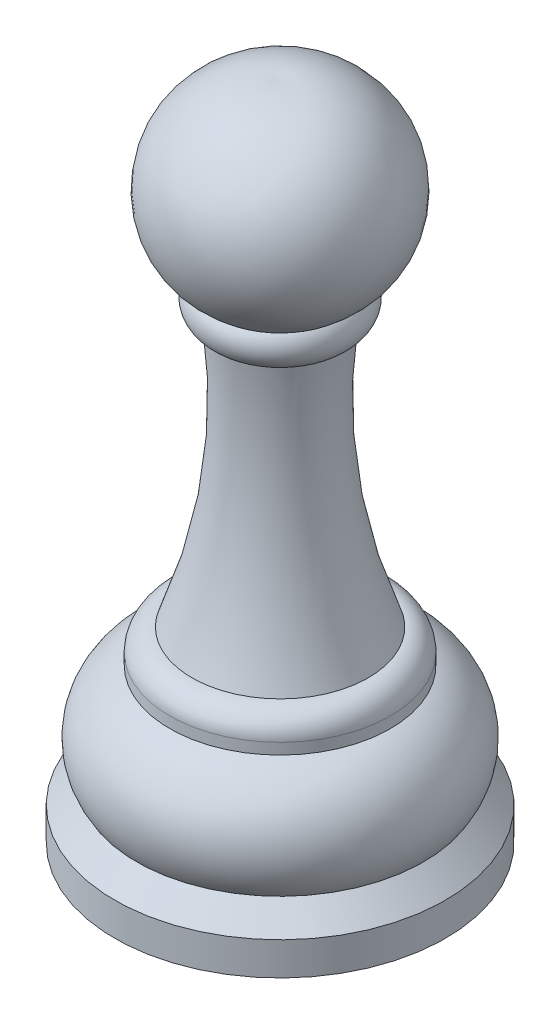
ISO-10303-21;
HEADER;
FILE_DESCRIPTION(('STEP AP214'),'2;1');
FILE_NAME('part.step','',(''),(''),'','','');
FILE_SCHEMA(('AUTOMOTIVE_DESIGN { 1 0 10303 214 1 1 1 1 }'));
ENDSEC;
DATA;
#1=APPLICATION_CONTEXT('core data for automotive mechanical design processes');
#2=APPLICATION_PROTOCOL_DEFINITION('international standard','automotive_design',2000,#1);
#3=PRODUCT_CONTEXT('',#1,'mechanical');
#4=PRODUCT('Part','Part','',(#3));
#5=PRODUCT_RELATED_PRODUCT_CATEGORY('part','',(#4));
#6=PRODUCT_DEFINITION_FORMATION('','',#4);
#7=PRODUCT_DEFINITION_CONTEXT('part definition',#1,'design');
#8=PRODUCT_DEFINITION('design','',#6,#7);
#9=PRODUCT_DEFINITION_SHAPE('','',#8);
#10=(LENGTH_UNIT() NAMED_UNIT(*) SI_UNIT(.MILLI.,.METRE.));
#11=(NAMED_UNIT(*) PLANE_ANGLE_UNIT() SI_UNIT($,.RADIAN.));
#12=(NAMED_UNIT(*) SI_UNIT($,.STERADIAN.) SOLID_ANGLE_UNIT());
#13=UNCERTAINTY_MEASURE_WITH_UNIT(LENGTH_MEASURE(1.E-05),#10,'distance_accuracy_value','');
#14=(GEOMETRIC_REPRESENTATION_CONTEXT(3) GLOBAL_UNCERTAINTY_ASSIGNED_CONTEXT((#13)) GLOBAL_UNIT_ASSIGNED_CONTEXT((#10,
#11,#12)) REPRESENTATION_CONTEXT('',''));
#15=CARTESIAN_POINT('',(0.,0.,0.));
#16=DIRECTION('',(0.,0.,1.));
#17=DIRECTION('',(1.,0.,0.));
#18=AXIS2_PLACEMENT_3D('',#15,#16,#17);
#19=CARTESIAN_POINT('',(0.,0.,0.));
#20=DIRECTION('',(0.,-1.,0.));
#21=DIRECTION('',(0.,0.,-1.));
#22=AXIS2_PLACEMENT_3D('',#19,#20,#21);
#23=PLANE('',#22);
#24=CARTESIAN_POINT('',(0.,0.,0.));
#25=DIRECTION('',(0.,-1.,0.));
#26=DIRECTION('',(0.,0.,-1.));
#27=AXIS2_PLACEMENT_3D('',#24,#25,#26);
#28=CIRCLE('',#27,15.);
#29=CARTESIAN_POINT('',(0.,0.,-15.));
#30=VERTEX_POINT('',#29);
#31=EDGE_CURVE('E11',#30,#30,#28,.T.);
#32=ORIENTED_EDGE('',*,*,#31,.T.);
#33=EDGE_LOOP('',(#32));
#34=FACE_BOUND('',#33,.T.);
#35=ADVANCED_FACE('F39',(#34),#23,.T.);
#36=CARTESIAN_POINT('',(0.,0.,0.));
#37=DIRECTION('',(0.,-1.,0.));
#38=DIRECTION('',(0.,0.,-1.));
#39=AXIS2_PLACEMENT_3D('',#36,#37,#38);
#40=CYLINDRICAL_SURFACE('',#39,15.);
#41=CARTESIAN_POINT('',(0.,3.,0.));
#42=DIRECTION('',(0.,-1.,0.));
#43=DIRECTION('',(0.,0.,-1.));
#44=AXIS2_PLACEMENT_3D('',#41,#42,#43);
#45=CIRCLE('',#44,15.);
#46=CARTESIAN_POINT('',(0.,3.,-15.));
#47=VERTEX_POINT('',#46);
#48=EDGE_CURVE('E44',#47,#47,#45,.T.);
#49=ORIENTED_EDGE('',*,*,#48,.T.);
#50=EDGE_LOOP('',(#49));
#51=FACE_BOUND('',#50,.T.);
#52=ORIENTED_EDGE('',*,*,#31,.F.);
#53=EDGE_LOOP('',(#52));
#54=FACE_BOUND('',#53,.T.);
#55=ADVANCED_FACE('F78',(#51,#54),#40,.T.);
#56=CARTESIAN_POINT('',(0.,3.,0.));
#57=DIRECTION('',(0.,-1.,0.));
#58=DIRECTION('',(0.,0.,-1.));
#59=AXIS2_PLACEMENT_3D('',#56,#57,#58);
#60=CONICAL_SURFACE('',#59,15.,0.785398163397448);
#61=CARTESIAN_POINT('',(0.,5.,0.));
#62=DIRECTION('',(0.,-1.,0.));
#63=DIRECTION('',(0.,0.,-1.));
#64=AXIS2_PLACEMENT_3D('',#61,#62,#63);
#65=CIRCLE('',#64,13.);
#66=CARTESIAN_POINT('',(0.,5.,-13.));
#67=VERTEX_POINT('',#66);
#68=EDGE_CURVE('E73',#67,#67,#65,.T.);
#69=ORIENTED_EDGE('',*,*,#68,.T.);
#70=EDGE_LOOP('',(#69));
#71=FACE_BOUND('',#70,.T.);
#72=ORIENTED_EDGE('',*,*,#48,.F.);
#73=EDGE_LOOP('',(#72));
#74=FACE_BOUND('',#73,.T.);
#75=ADVANCED_FACE('F80',(#71,#74),#60,.T.);
#76=CARTESIAN_POINT('',(0.,8.31380661428568,0.));
#77=DIRECTION('',(0.,-1.,0.));
#78=DIRECTION('',(0.,0.,-1.));
#79=AXIS2_PLACEMENT_3D('',#76,#77,#78);
#80=TOROIDAL_SURFACE('',#79,7.99813177671417,6.);
#81=CARTESIAN_POINT('',(0.,13.97,0.));
#82=DIRECTION('',(0.,-1.,0.));
#83=DIRECTION('',(0.,0.,-1.));
#84=AXIS2_PLACEMENT_3D('',#81,#82,#83);
#85=CIRCLE('',#84,10.);
#86=CARTESIAN_POINT('',(0.,13.97,-10.));
#87=VERTEX_POINT('',#86);
#88=EDGE_CURVE('E66',#87,#87,#85,.T.);
#89=ORIENTED_EDGE('',*,*,#88,.T.);
#90=EDGE_LOOP('',(#89));
#91=FACE_BOUND('',#90,.T.);
#92=ORIENTED_EDGE('',*,*,#68,.F.);
#93=EDGE_LOOP('',(#92));
#94=FACE_BOUND('',#93,.T.);
#95=ADVANCED_FACE('F83',(#91,#94),#80,.T.);
#96=CARTESIAN_POINT('',(0.,0.,0.));
#97=DIRECTION('',(0.,-1.,0.));
#98=DIRECTION('',(0.,0.,-1.));
#99=AXIS2_PLACEMENT_3D('',#96,#97,#98);
#100=CYLINDRICAL_SURFACE('',#99,10.);
#101=CARTESIAN_POINT('',(0.,14.97,0.));
#102=DIRECTION('',(0.,-1.,0.));
#103=DIRECTION('',(0.,0.,-1.));
#104=AXIS2_PLACEMENT_3D('',#101,#102,#103);
#105=CIRCLE('',#104,10.);
#106=CARTESIAN_POINT('',(0.,14.97,-10.));
#107=VERTEX_POINT('',#106);
#108=EDGE_CURVE('E64',#107,#107,#105,.T.);
#109=ORIENTED_EDGE('',*,*,#108,.T.);
#110=EDGE_LOOP('',(#109));
#111=FACE_BOUND('',#110,.T.);
#112=ORIENTED_EDGE('',*,*,#88,.F.);
#113=EDGE_LOOP('',(#112));
#114=FACE_BOUND('',#113,.T.);
#115=ADVANCED_FACE('F88',(#111,#114),#100,.T.);
#116=CARTESIAN_POINT('',(0.,14.97,0.));
#117=DIRECTION('',(0.,-1.,0.));
#118=DIRECTION('',(0.,0.,-1.));
#119=AXIS2_PLACEMENT_3D('',#116,#117,#118);
#120=TOROIDAL_SURFACE('',#119,8.,2.);
#121=CARTESIAN_POINT('',(0.,16.97,0.));
#122=DIRECTION('',(0.,-1.,0.));
#123=DIRECTION('',(0.,0.,-1.));
#124=AXIS2_PLACEMENT_3D('',#121,#122,#123);
#125=CIRCLE('',#124,8.);
#126=CARTESIAN_POINT('',(0.,16.97,-8.));
#127=VERTEX_POINT('',#126);
#128=EDGE_CURVE('E58',#127,#127,#125,.T.);
#129=ORIENTED_EDGE('',*,*,#128,.T.);
#130=EDGE_LOOP('',(#129));
#131=FACE_BOUND('',#130,.T.);
#132=ORIENTED_EDGE('',*,*,#108,.F.);
#133=EDGE_LOOP('',(#132));
#134=FACE_BOUND('',#133,.T.);
#135=ADVANCED_FACE('F123',(#131,#134),#120,.T.);
#136=CARTESIAN_POINT('',(0.,35.0019065796665,0.));
#137=DIRECTION('',(0.,-1.,0.));
#138=DIRECTION('',(0.,0.,-1.));
#139=AXIS2_PLACEMENT_3D('',#136,#137,#138);
#140=TOROIDAL_SURFACE('',#139,54.635290768925,50.);
#141=CARTESIAN_POINT('',(0.,41.03,0.));
#142=DIRECTION('',(0.,-1.,0.));
#143=DIRECTION('',(0.,0.,-1.));
#144=AXIS2_PLACEMENT_3D('',#141,#142,#143);
#145=CIRCLE('',#144,5.);
#146=CARTESIAN_POINT('',(0.,41.03,-5.));
#147=VERTEX_POINT('',#146);
#148=EDGE_CURVE('E60',#147,#147,#145,.T.);
#149=ORIENTED_EDGE('',*,*,#148,.T.);
#150=EDGE_LOOP('',(#149));
#151=FACE_BOUND('',#150,.T.);
#152=ORIENTED_EDGE('',*,*,#128,.F.);
#153=EDGE_LOOP('',(#152));
#154=FACE_BOUND('',#153,.T.);
#155=ADVANCED_FACE('F131',(#151,#154),#140,.F.);
#156=CARTESIAN_POINT('',(0.,42.966609004825,0.));
#157=DIRECTION('',(0.,-1.,0.));
#158=DIRECTION('',(0.,0.,-1.));
#159=AXIS2_PLACEMENT_3D('',#156,#157,#158);
#160=TOROIDAL_SURFACE('',#159,4.50045464427059,2.);
#161=CARTESIAN_POINT('',(0.,44.29,0.));
#162=DIRECTION('',(0.,-1.,0.));
#163=DIRECTION('',(0.,0.,-1.));
#164=AXIS2_PLACEMENT_3D('',#161,#162,#163);
#165=CIRCLE('',#164,6.);
#166=CARTESIAN_POINT('',(0.,44.29,-6.));
#167=VERTEX_POINT('',#166);
#168=EDGE_CURVE('E54',#167,#167,#165,.T.);
#169=ORIENTED_EDGE('',*,*,#168,.T.);
#170=EDGE_LOOP('',(#169));
#171=FACE_BOUND('',#170,.T.);
#172=ORIENTED_EDGE('',*,*,#148,.F.);
#173=EDGE_LOOP('',(#172));
#174=FACE_BOUND('',#173,.T.);
#175=ADVANCED_FACE('F51',(#171,#174),#160,.T.);
#176=CARTESIAN_POINT('',(0.,51.3270170273711,-0.858247916666662));
#177=DIRECTION('',(-1.,0.,0.));
#178=DIRECTION('',(0.,0.,-1.));
#179=AXIS2_PLACEMENT_3D('',#176,#177,#178);
#180=CIRCLE('',#179,8.71534411999741);
#181=TRIMMED_CURVE('',#180,(PARAMETER_VALUE(-1.6694316905533)),
(PARAMETER_VALUE(1.6694316905533)),.T.,.PARAMETER.);
#182=CARTESIAN_POINT('',(0.,51.3270170273711,0.));
#183=DIRECTION('',(0.,-1.,0.));
#184=AXIS1_PLACEMENT('',#182,#183);
#185=SURFACE_OF_REVOLUTION('',#181,#184);
#186=CARTESIAN_POINT('',(0.,60.,0.));
#187=VERTEX_POINT('',#186);
#188=VERTEX_LOOP('',#187);
#189=FACE_BOUND('',#188,.T.);
#190=ORIENTED_EDGE('',*,*,#168,.F.);
#191=EDGE_LOOP('',(#190));
#192=FACE_BOUND('',#191,.T.);
#193=ADVANCED_FACE('F48',(#189,#192),#185,.T.);
#194=CLOSED_SHELL('',(#35,#55,#75,#95,#115,#135,#155,#175,#193));
#195=MANIFOLD_SOLID_BREP('B2',#194);
#196=ADVANCED_BREP_SHAPE_REPRESENTATION('',(#18,#195),#14);
#197=SHAPE_DEFINITION_REPRESENTATION(#9,#196);
ENDSEC;
END-ISO-10303-21;
